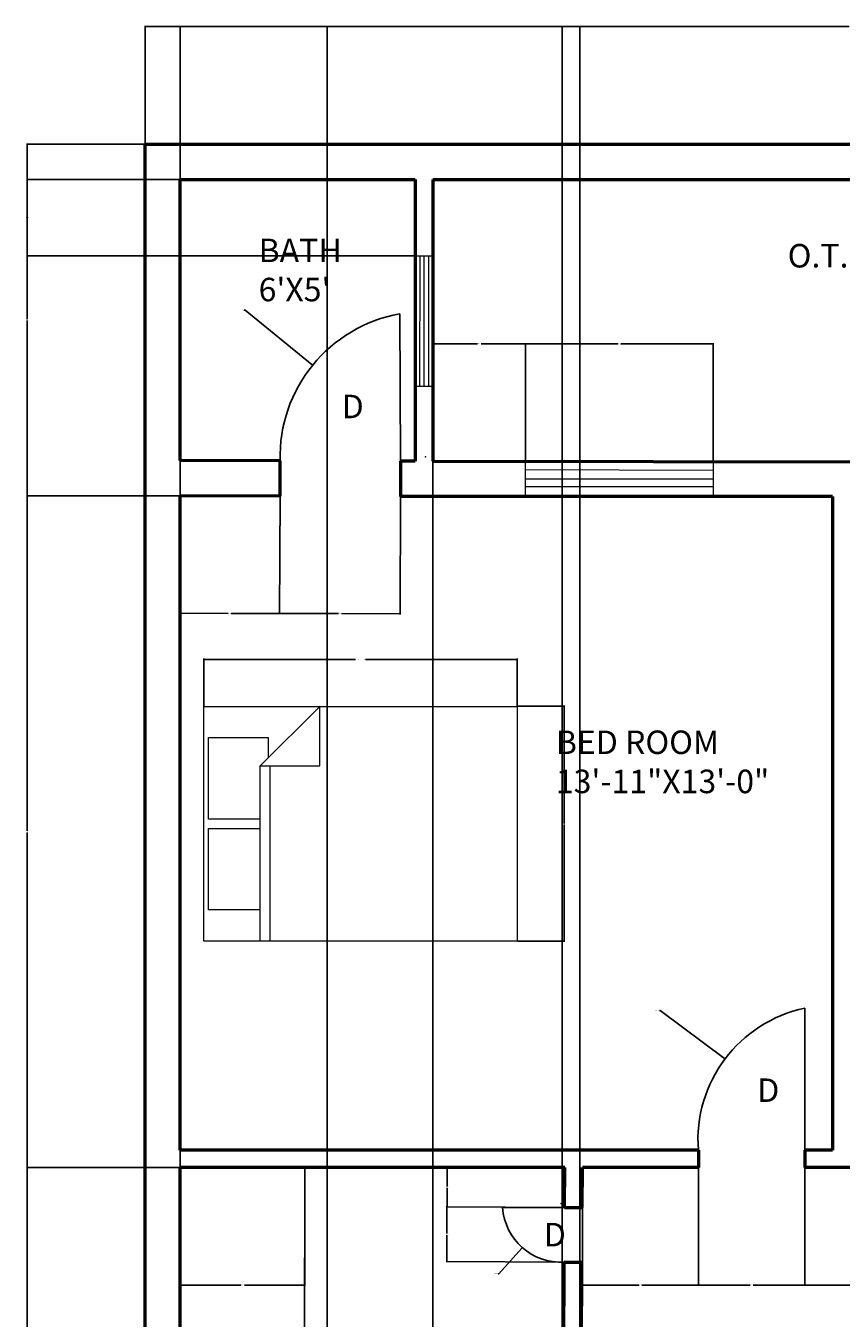
# Model space of a CAD drawing. Units: inches. Extents: x 2341 to 2761, y 2129 to 2789.
# Tile 3 of 4: x 2341 to 2549, y 2459 to 2789. Entities that reach past the tile are written whole.
import ezdxf

# ---------------------------------------------------------------- set-up
doc = ezdxf.new("R2010")
doc.units = ezdxf.units.IN
for name, color, linetype, lineweight in [('A-ANNO-DIMS', 2, 'Continuous', 18), ('A-ANNO-TEXT', 7, 'Continuous', 18), ('A-AREA-IDEN', 7, 'Continuous', 25), ('A-DOOR', 3, 'Continuous', 25), ('A-FLOR-FIXT', 9, 'Continuous', 25), ('A-FURN', 8, 'Continuous', 18), ('A-GLAZ', 4, 'Continuous', 18), ('A-WALL', 7, 'Continuous', 50)]:
    doc.layers.add(name, color=color, linetype=linetype, lineweight=lineweight)
doc.styles.get("Standard").update_dxf_attribs({"font": 'arial.ttf'})
doc.dimstyles.get("Standard").update_dxf_attribs({"dimtxt": 0.18, "dimasz": 0.18, "dimexe": 0.18, "dimexo": 0.0625, "dimgap": 0.09, "dimtad": 0, "dimtih": 1, "dimtoh": 1, "dimdec": 4, "dimzin": 0, "dimdsep": 46, "dimtxsty": 'Standard', "dimcen": 0.09, "dimadec": 0, "dimazin": 0, "dimtfac": 1, "dimtdec": 4, "dimtofl": 0, "dimtmove": 0, "dimatfit": 3, "dimfxl": 1, "dimtolj": 1, "dimtzin": 0, "dimarcsym": 0})

# ---------------------------------------------------------------- blocks, each defined once
blk = doc.blocks.new('Bed - Queen')
for p, q in [((0, -80.00003), (0, 0)), ((0, 0), (59.99999, 0)), ((59.99999, 0), (59.99999, -80.00003)), ((7.99999, -1.2), (28.79998, -1.2)), ((7.99999, -14.4), (7.99999, -1.2)), ((28.79998, -1.2), (28.79998, -14.4)), ((31.19999, -1.2), (51.99999, -1.2)), ((31.19999, -14.4), (31.19999, -1.2)), ((51.99999, -1.2), (51.99999, -16.4)), ((0, -14.4), (44.8, -14.4)), ((59.99999, -29.6), (44.8, -14.4)), ((44.8, -14.4), (44.8, -29.6)), ((51.99999, -16.4), (46.79936, -16.4)), ((44.8, -16.8), (0, -16.8)), ((44.8, -29.6), (59.99999, -29.6)), ((59.99999, -80.00003), (0, -80.00003))]:
    blk.add_line(p, q)
blk = doc.blocks.new('WIN-33IN-NARROW')
for p, q in [((0, 3.43), (33.34, 3.43)), ((0, 2.27), (33.34, 2.27)), ((0, 1.23), (33.34, 1.12))]:
    blk.add_line(p, q)
blk.add_lwpolyline([(0, 4.54), (33.34, 4.54), (33.34, 0), (0, 0)], close=True)
blk = doc.blocks.new('*D7')
at = {"layer": 'A-ANNO-DIMS', "color": 0, "lineweight": -2, "transparency": 16777216}
for p, q in [((2386.27, 2615.54), (2386.27, 2627.66)), ((2386.45, 2627.48), (2424.97, 2627.48)), ((2466.09, 2627.48), (2427.57, 2627.48)), ((2466.27, 2615.54), (2466.27, 2627.66))]:
    blk.add_line(p, q, dxfattribs=at)
at = {"layer": 'A-ANNO-DIMS', "color": 0, "transparency": 16777216}
for points in [[(2386.45, 2627.51), (2386.45, 2627.45), (2386.27, 2627.48)], [(2466.09, 2627.51), (2466.09, 2627.45), (2466.27, 2627.48)]]:
    blk.add_solid(points, dxfattribs=at)
at = {"layer": 'Defpoints', "color": 0, "transparency": 16777216}
for p in [(2386.27, 2627.48), (2386.27, 2615.48), (2466.27, 2615.48)]:
    blk.add_point(p, dxfattribs=at)
at = {"layer": 'A-ANNO-DIMS', "color": 0, "transparency": 16777216, "insert": (2426.27, 2627.48), "char_height": 0.18, "attachment_point": 5}
blk.add_mtext('\\A1;QUEEN BED 80 TYP.', dxfattribs=at)
blk = doc.blocks.new('*D8')
at = {"layer": 'A-ANNO-DIMS', "color": 0, "lineweight": -2, "transparency": 16777216}
for p, q in [((2466.33, 2615.48), (2478.45, 2615.48)), ((2478.27, 2615.3), (2478.27, 2585.66)), ((2478.27, 2555.66), (2478.27, 2585.3)), ((2466.33, 2555.48), (2478.45, 2555.48))]:
    blk.add_line(p, q, dxfattribs=at)
at = {"layer": 'A-ANNO-DIMS', "color": 0, "transparency": 16777216}
for points in [[(2478.24, 2615.3), (2478.3, 2615.3), (2478.27, 2615.48)], [(2478.24, 2555.66), (2478.3, 2555.66), (2478.27, 2555.48)]]:
    blk.add_solid(points, dxfattribs=at)
at = {"layer": 'Defpoints', "color": 0, "transparency": 16777216}
for p in [(2466.27, 2615.48), (2478.27, 2615.48), (2466.27, 2555.48)]:
    blk.add_point(p, dxfattribs=at)
at = {"layer": 'A-ANNO-DIMS', "color": 0, "transparency": 16777216, "insert": (2478.27, 2585.48), "char_height": 0.18, "attachment_point": 5}
blk.add_mtext('\\A1;60 TYP.', dxfattribs=at)
blk = doc.blocks.new('*D11')
at = {"layer": 'A-ANNO-DIMS', "color": 0, "lineweight": -2, "transparency": 16777216}
for p, q in [((2371.24, 2759.18), (2371.24, 2789.36)), ((2371.42, 2789.18), (2550.95, 2789.18)), ((2731.06, 2789.18), (2551.53, 2789.18)), ((2731.24, 2759.18), (2731.24, 2789.36))]:
    blk.add_line(p, q, dxfattribs=at)
at = {"layer": 'A-ANNO-DIMS', "color": 0, "transparency": 16777216}
for points in [[(2371.42, 2789.21), (2371.42, 2789.15), (2371.24, 2789.18)], [(2731.06, 2789.21), (2731.06, 2789.15), (2731.24, 2789.18)]]:
    blk.add_solid(points, dxfattribs=at)
at = {"layer": 'Defpoints', "color": 0, "transparency": 16777216}
for p in [(2731.24, 2789.18), (2371.24, 2759.12), (2731.24, 2759.12)]:
    blk.add_point(p, dxfattribs=at)
at = {"layer": 'A-ANNO-DIMS', "color": 0, "transparency": 16777216, "insert": (2551.24, 2789.18), "char_height": 0.18, "attachment_point": 5}
blk.add_mtext('\\A1;360', dxfattribs=at)
blk = doc.blocks.new('*D14')
at = {"layer": 'A-ANNO-DIMS', "color": 0, "lineweight": -2, "transparency": 16777216}
for p, q in [((2380.18, 2497.6), (2341.01, 2497.6)), ((2341.19, 2497.42), (2341.19, 2419.77)), ((2341.19, 2341.76), (2341.19, 2419.4)), ((2380.18, 2341.58), (2341.01, 2341.58))]:
    blk.add_line(p, q, dxfattribs=at)
at = {"layer": 'A-ANNO-DIMS', "color": 0, "transparency": 16777216}
for points in [[(2341.16, 2497.42), (2341.22, 2497.42), (2341.19, 2497.6)], [(2341.16, 2341.76), (2341.22, 2341.76), (2341.19, 2341.58)]]:
    blk.add_solid(points, dxfattribs=at)
at = {"layer": 'Defpoints', "color": 0, "transparency": 16777216}
for p in [(2341.19, 2497.6), (2380.24, 2497.6), (2380.24, 2341.58)]:
    blk.add_point(p, dxfattribs=at)
at = {"layer": 'A-ANNO-DIMS', "color": 0, "transparency": 16777216, "insert": (2341.19, 2419.59), "char_height": 0.18, "attachment_point": 5}
blk.add_mtext('\\A1;156.02', dxfattribs=at)
blk = doc.blocks.new('*D15')
at = {"layer": 'A-ANNO-DIMS', "color": 0, "lineweight": -2, "transparency": 16777216}
for p, q in [((2380.18, 2669.3), (2341.01, 2669.3)), ((2341.19, 2669.12), (2341.19, 2583.63)), ((2341.19, 2497.78), (2341.19, 2583.27)), ((2380.18, 2497.6), (2341.01, 2497.6))]:
    blk.add_line(p, q, dxfattribs=at)
at = {"layer": 'A-ANNO-DIMS', "color": 0, "transparency": 16777216}
for points in [[(2341.16, 2669.12), (2341.22, 2669.12), (2341.19, 2669.3)], [(2341.16, 2497.78), (2341.22, 2497.78), (2341.19, 2497.6)]]:
    blk.add_solid(points, dxfattribs=at)
at = {"layer": 'Defpoints', "color": 0, "transparency": 16777216}
for p in [(2341.19, 2669.3), (2380.24, 2669.3), (2380.24, 2497.6)]:
    blk.add_point(p, dxfattribs=at)
at = {"layer": 'A-ANNO-DIMS', "color": 0, "transparency": 16777216, "insert": (2341.19, 2583.45), "char_height": 0.18, "attachment_point": 5}
blk.add_mtext('\\A1;171.7', dxfattribs=at)
blk = doc.blocks.new('*D16')
at = {"layer": 'A-ANNO-DIMS', "color": 0, "lineweight": -2, "transparency": 16777216}
for p, q in [((2371.18, 2759.12), (2341.01, 2759.12)), ((2341.19, 2758.94), (2341.19, 2714.39)), ((2341.19, 2669.48), (2341.19, 2714.03)), ((2380.18, 2669.3), (2341.01, 2669.3))]:
    blk.add_line(p, q, dxfattribs=at)
at = {"layer": 'A-ANNO-DIMS', "color": 0, "transparency": 16777216}
for points in [[(2341.16, 2758.94), (2341.22, 2758.94), (2341.19, 2759.12)], [(2341.16, 2669.48), (2341.22, 2669.48), (2341.19, 2669.3)]]:
    blk.add_solid(points, dxfattribs=at)
at = {"layer": 'Defpoints', "color": 0, "transparency": 16777216}
for p in [(2341.19, 2759.12), (2371.24, 2759.12), (2380.24, 2669.3)]:
    blk.add_point(p, dxfattribs=at)
at = {"layer": 'A-ANNO-DIMS', "color": 0, "transparency": 16777216, "insert": (2341.19, 2714.21), "char_height": 0.18, "attachment_point": 5}
blk.add_mtext('\\A1;89.82', dxfattribs=at)
blk = doc.blocks.new('*D17')
at = {"layer": 'A-ANNO-DIMS', "color": 0, "lineweight": -2, "transparency": 16777216}
for p, q in [((2444.74, 2750.05), (2444.74, 2128.92)), ((2658.39, 2749.97), (2658.39, 2128.92)), ((2444.92, 2129.1), (2551.1, 2129.1)), ((2658.21, 2129.1), (2552.03, 2129.1))]:
    blk.add_line(p, q, dxfattribs=at)
at = {"layer": 'A-ANNO-DIMS', "color": 0, "transparency": 16777216}
for points in [[(2444.92, 2129.13), (2444.92, 2129.07), (2444.74, 2129.1)], [(2658.21, 2129.13), (2658.21, 2129.07), (2658.39, 2129.1)]]:
    blk.add_solid(points, dxfattribs=at)
at = {"layer": 'Defpoints', "color": 0, "transparency": 16777216}
for p in [(2444.74, 2750.12), (2658.39, 2750.04), (2658.39, 2129.1)]:
    blk.add_point(p, dxfattribs=at)
at = {"layer": 'A-ANNO-DIMS', "color": 0, "transparency": 16777216, "insert": (2551.56, 2129.1), "char_height": 0.18, "attachment_point": 5}
blk.add_mtext('\\A1;213.65', dxfattribs=at)
blk = doc.blocks.new('*D28')
at = {"layer": 'A-ANNO-DIMS', "color": 0, "lineweight": -2, "transparency": 16777216}
for p, q in [((2477.74, 2346.18), (2477.74, 2789.36)), ((2477.92, 2789.18), (2479.73, 2789.18)), ((2482.06, 2789.18), (2480.25, 2789.18)), ((2482.24, 2346.16), (2482.24, 2789.36))]:
    blk.add_line(p, q, dxfattribs=at)
at = {"layer": 'A-ANNO-DIMS', "color": 0, "transparency": 16777216}
for points in [[(2477.92, 2789.21), (2477.92, 2789.15), (2477.74, 2789.18)], [(2482.06, 2789.21), (2482.06, 2789.15), (2482.24, 2789.18)]]:
    blk.add_solid(points, dxfattribs=at)
at = {"layer": 'Defpoints', "color": 0, "transparency": 16777216}
for p in [(2482.24, 2789.18), (2477.74, 2346.12), (2482.24, 2346.1)]:
    blk.add_point(p, dxfattribs=at)
at = {"layer": 'A-ANNO-DIMS', "color": 0, "transparency": 16777216, "insert": (2479.99, 2789.18), "char_height": 0.18, "attachment_point": 5}
blk.add_mtext('\\A1;4.5', dxfattribs=at)
blk = doc.blocks.new('*D29')
at = {"layer": 'A-ANNO-DIMS', "color": 0, "lineweight": -2, "transparency": 16777216}
for p, q in [((2371.24, 2759.06), (2371.24, 2128.92)), ((2380.24, 2750.06), (2380.24, 2128.92)), ((2371.42, 2129.1), (2375.59, 2129.1)), ((2380.06, 2129.1), (2375.89, 2129.1))]:
    blk.add_line(p, q, dxfattribs=at)
at = {"layer": 'A-ANNO-DIMS', "color": 0, "transparency": 16777216}
for points in [[(2371.42, 2129.13), (2371.42, 2129.07), (2371.24, 2129.1)], [(2380.06, 2129.13), (2380.06, 2129.07), (2380.24, 2129.1)]]:
    blk.add_solid(points, dxfattribs=at)
at = {"layer": 'Defpoints', "color": 0, "transparency": 16777216}
for p in [(2371.24, 2759.12), (2380.24, 2750.12), (2380.24, 2129.1)]:
    blk.add_point(p, dxfattribs=at)
at = {"layer": 'A-ANNO-DIMS', "color": 0, "transparency": 16777216, "insert": (2375.74, 2129.1), "char_height": 0.18, "attachment_point": 5}
blk.add_mtext('\\A1;9', dxfattribs=at)
blk = doc.blocks.new('*D31')
at = {"layer": 'A-ANNO-DIMS', "color": 0, "lineweight": -2, "transparency": 16777216}
for p, q in [((2444.74, 2678.18), (2444.78, 2708.32)), ((2444.96, 2708.14), (2456.13, 2708.12)), ((2468.24, 2708.11), (2457.06, 2708.12)), ((2468.39, 2678.15), (2468.42, 2708.29))]:
    blk.add_line(p, q, dxfattribs=at)
at = {"layer": 'A-ANNO-DIMS', "color": 0, "transparency": 16777216}
for points in [[(2444.96, 2708.17), (2444.96, 2708.11), (2444.78, 2708.14)], [(2468.24, 2708.14), (2468.24, 2708.08), (2468.42, 2708.11)]]:
    blk.add_solid(points, dxfattribs=at)
at = {"layer": 'Defpoints', "color": 0, "transparency": 16777216}
for p in [(2468.42, 2708.11), (2444.74, 2678.12), (2468.39, 2678.09)]:
    blk.add_point(p, dxfattribs=at)
at = {"layer": 'A-ANNO-DIMS', "color": 0, "transparency": 16777216, "insert": (2456.6, 2708.12), "char_height": 0.18, "attachment_point": 5}
blk.add_mtext('\\A1;23.643', dxfattribs=at)
blk = doc.blocks.new('*D32')
at = {"layer": 'A-ANNO-DIMS', "color": 0, "lineweight": -2, "transparency": 16777216}
for p, q in [((2468.39, 2678.15), (2468.39, 2708.29)), ((2468.57, 2708.11), (2491.95, 2708.11)), ((2516.12, 2708.11), (2492.74, 2708.11)), ((2516.3, 2678.15), (2516.3, 2708.29))]:
    blk.add_line(p, q, dxfattribs=at)
at = {"layer": 'A-ANNO-DIMS', "color": 0, "transparency": 16777216}
for points in [[(2468.57, 2708.14), (2468.57, 2708.08), (2468.39, 2708.11)], [(2516.12, 2708.14), (2516.12, 2708.08), (2516.3, 2708.11)]]:
    blk.add_solid(points, dxfattribs=at)
at = {"layer": 'Defpoints', "color": 0, "transparency": 16777216}
for p in [(2516.3, 2708.11), (2468.39, 2678.09), (2516.3, 2678.09)]:
    blk.add_point(p, dxfattribs=at)
at = {"layer": 'A-ANNO-DIMS', "color": 0, "transparency": 16777216, "insert": (2492.34, 2708.11), "char_height": 0.18, "attachment_point": 5}
blk.add_mtext('\\A1;47.92', dxfattribs=at)
blk = doc.blocks.new('*D33')
at = {"layer": 'A-ANNO-DIMS', "color": 0, "lineweight": -2, "transparency": 16777216}
for p, q in [((2380.24, 2346.14), (2380.24, 2789.36)), ((2380.42, 2789.18), (2398.59, 2789.18)), ((2417.55, 2789.18), (2399.38, 2789.18)), ((2417.73, 2346.19), (2417.73, 2789.36))]:
    blk.add_line(p, q, dxfattribs=at)
at = {"layer": 'A-ANNO-DIMS', "color": 0, "transparency": 16777216}
for points in [[(2380.42, 2789.21), (2380.42, 2789.15), (2380.24, 2789.18)], [(2417.55, 2789.21), (2417.55, 2789.15), (2417.73, 2789.18)]]:
    blk.add_solid(points, dxfattribs=at)
at = {"layer": 'Defpoints', "color": 0, "transparency": 16777216}
for p in [(2417.73, 2789.18), (2380.24, 2346.08), (2417.73, 2346.13)]:
    blk.add_point(p, dxfattribs=at)
at = {"layer": 'A-ANNO-DIMS', "color": 0, "transparency": 16777216, "insert": (2398.99, 2789.18), "char_height": 0.18, "attachment_point": 5}
blk.add_mtext('\\A1;37.49', dxfattribs=at)
blk = doc.blocks.new('*D36')
at = {"layer": 'A-ANNO-DIMS', "color": 0, "lineweight": -2, "transparency": 16777216}
for p, q in [((2440.18, 2750.12), (2341.01, 2750.12)), ((2341.19, 2749.94), (2341.19, 2740.52)), ((2341.19, 2730.74), (2341.19, 2740.16)), ((2440.14, 2730.56), (2341.01, 2730.56))]:
    blk.add_line(p, q, dxfattribs=at)
at = {"layer": 'A-ANNO-DIMS', "color": 0, "transparency": 16777216}
for points in [[(2341.16, 2749.94), (2341.22, 2749.94), (2341.19, 2750.12)], [(2341.16, 2730.74), (2341.22, 2730.74), (2341.19, 2730.56)]]:
    blk.add_solid(points, dxfattribs=at)
at = {"layer": 'Defpoints', "color": 0, "transparency": 16777216}
for p in [(2341.19, 2750.12), (2440.24, 2750.12), (2440.2, 2730.56)]:
    blk.add_point(p, dxfattribs=at)
at = {"layer": 'A-ANNO-DIMS', "color": 0, "transparency": 16777216, "insert": (2341.19, 2740.34), "char_height": 0.18, "attachment_point": 5}
blk.add_mtext('\\A1;19.554', dxfattribs=at)
blk = doc.blocks.new('*D37')
at = {"layer": 'A-ANNO-DIMS', "color": 0, "lineweight": -2, "transparency": 16777216}
for p, q in [((2380.24, 2669.24), (2380.15, 2639.1)), ((2405.71, 2669.16), (2405.62, 2639.02)), ((2380.33, 2639.28), (2392.49, 2639.24)), ((2405.44, 2639.2), (2393.28, 2639.24))]:
    blk.add_line(p, q, dxfattribs=at)
at = {"layer": 'A-ANNO-DIMS', "color": 0, "transparency": 16777216}
for points in [[(2380.33, 2639.31), (2380.33, 2639.25), (2380.15, 2639.28)], [(2405.44, 2639.23), (2405.44, 2639.17), (2405.62, 2639.2)]]:
    blk.add_solid(points, dxfattribs=at)
at = {"layer": 'Defpoints', "color": 0, "transparency": 16777216}
for p in [(2380.24, 2669.3), (2405.71, 2669.22), (2380.15, 2639.28)]:
    blk.add_point(p, dxfattribs=at)
at = {"layer": 'A-ANNO-DIMS', "color": 0, "transparency": 16777216, "insert": (2392.89, 2639.24), "char_height": 0.18, "attachment_point": 5}
blk.add_mtext('\\A1;25.47', dxfattribs=at)
blk = doc.blocks.new('*D38')
at = {"layer": 'A-ANNO-DIMS', "color": 0, "lineweight": -2, "transparency": 16777216}
for p, q in [((2405.71, 2669.16), (2405.62, 2639.02)), ((2436.5, 2669.07), (2436.41, 2638.93)), ((2405.8, 2639.2), (2420.62, 2639.16)), ((2436.23, 2639.11), (2421.41, 2639.16))]:
    blk.add_line(p, q, dxfattribs=at)
at = {"layer": 'A-ANNO-DIMS', "color": 0, "transparency": 16777216}
for points in [[(2405.8, 2639.23), (2405.8, 2639.17), (2405.62, 2639.2)], [(2436.23, 2639.14), (2436.23, 2639.08), (2436.41, 2639.11)]]:
    blk.add_solid(points, dxfattribs=at)
at = {"layer": 'Defpoints', "color": 0, "transparency": 16777216}
for p in [(2405.71, 2669.22), (2436.5, 2669.13), (2405.62, 2639.2)]:
    blk.add_point(p, dxfattribs=at)
at = {"layer": 'A-ANNO-DIMS', "color": 0, "transparency": 16777216, "insert": (2421.02, 2639.16), "char_height": 0.18, "attachment_point": 5}
blk.add_mtext('\\A1;30.79', dxfattribs=at)
blk = doc.blocks.new('*D43')
at = {"layer": 'A-ANNO-DIMS', "color": 0, "lineweight": -2, "transparency": 16777216}
for p, q in [((2482.91, 2497.53), (2482.91, 2467.4)), ((2512.53, 2497.53), (2512.53, 2467.4)), ((2483.09, 2467.58), (2497.33, 2467.58)), ((2512.35, 2467.58), (2498.11, 2467.58))]:
    blk.add_line(p, q, dxfattribs=at)
at = {"layer": 'A-ANNO-DIMS', "color": 0, "transparency": 16777216}
for points in [[(2483.09, 2467.61), (2483.09, 2467.55), (2482.91, 2467.58)], [(2512.35, 2467.61), (2512.35, 2467.55), (2512.53, 2467.58)]]:
    blk.add_solid(points, dxfattribs=at)
at = {"layer": 'Defpoints', "color": 0, "transparency": 16777216}
for p in [(2482.91, 2497.6), (2512.53, 2497.6), (2482.91, 2467.58)]:
    blk.add_point(p, dxfattribs=at)
at = {"layer": 'A-ANNO-DIMS', "color": 0, "transparency": 16777216, "insert": (2497.72, 2467.58), "char_height": 0.18, "attachment_point": 5}
blk.add_mtext('\\A1;29.62', dxfattribs=at)
blk = doc.blocks.new('*D44')
at = {"layer": 'A-ANNO-DIMS', "color": 0, "lineweight": -2, "transparency": 16777216}
for p, q in [((2512.53, 2497.53), (2512.53, 2467.4)), ((2539.74, 2497.53), (2539.74, 2467.4)), ((2512.71, 2467.58), (2525.76, 2467.58)), ((2539.56, 2467.58), (2526.51, 2467.58))]:
    blk.add_line(p, q, dxfattribs=at)
at = {"layer": 'A-ANNO-DIMS', "color": 0, "transparency": 16777216}
for points in [[(2512.71, 2467.61), (2512.71, 2467.55), (2512.53, 2467.58)], [(2539.56, 2467.61), (2539.56, 2467.55), (2539.74, 2467.58)]]:
    blk.add_solid(points, dxfattribs=at)
at = {"layer": 'Defpoints', "color": 0, "transparency": 16777216}
for p in [(2512.53, 2497.6), (2539.74, 2497.6), (2512.53, 2467.58)]:
    blk.add_point(p, dxfattribs=at)
at = {"layer": 'A-ANNO-DIMS', "color": 0, "transparency": 16777216, "insert": (2526.13, 2467.58), "char_height": 0.18, "attachment_point": 5}
blk.add_mtext('\\A1;27.21', dxfattribs=at)
blk = doc.blocks.new('*D45')
at = {"layer": 'A-ANNO-DIMS', "color": 0, "lineweight": -2, "transparency": 16777216}
for p, q in [((2539.74, 2497.53), (2539.74, 2467.4)), ((2567.7, 2497.53), (2567.7, 2467.4)), ((2539.92, 2467.58), (2553.25, 2467.58)), ((2567.52, 2467.58), (2554.19, 2467.58))]:
    blk.add_line(p, q, dxfattribs=at)
at = {"layer": 'A-ANNO-DIMS', "color": 0, "transparency": 16777216}
for points in [[(2539.92, 2467.61), (2539.92, 2467.55), (2539.74, 2467.58)], [(2567.52, 2467.61), (2567.52, 2467.55), (2567.7, 2467.58)]]:
    blk.add_solid(points, dxfattribs=at)
at = {"layer": 'Defpoints', "color": 0, "transparency": 16777216}
for p in [(2539.74, 2497.6), (2567.7, 2497.6), (2539.74, 2467.58)]:
    blk.add_point(p, dxfattribs=at)
at = {"layer": 'A-ANNO-DIMS', "color": 0, "transparency": 16777216, "insert": (2553.72, 2467.58), "char_height": 0.18, "attachment_point": 5}
blk.add_mtext('\\A1;27.967', dxfattribs=at)
blk = doc.blocks.new('*D47')
at = {"layer": 'A-ANNO-DIMS', "color": 0, "lineweight": -2, "transparency": 16777216}
for p, q in [((2478.3, 2487.42), (2448.17, 2487.56)), ((2448.34, 2487.37), (2448.32, 2480.75)), ((2448.28, 2473.77), (2448.31, 2480.39)), ((2478.24, 2473.45), (2448.1, 2473.59))]:
    blk.add_line(p, q, dxfattribs=at)
at = {"layer": 'A-ANNO-DIMS', "color": 0, "transparency": 16777216}
for points in [[(2448.31, 2487.37), (2448.37, 2487.37), (2448.35, 2487.55)], [(2448.25, 2473.77), (2448.31, 2473.77), (2448.28, 2473.59)]]:
    blk.add_solid(points, dxfattribs=at)
at = {"layer": 'Defpoints', "color": 0, "transparency": 16777216}
for p in [(2448.35, 2487.55), (2478.37, 2487.42), (2478.3, 2473.45)]:
    blk.add_point(p, dxfattribs=at)
at = {"layer": 'A-ANNO-DIMS', "color": 0, "transparency": 16777216, "insert": (2448.31, 2480.57), "char_height": 0.18, "attachment_point": 5}
blk.add_mtext('\\A1;13.968', dxfattribs=at)
blk = doc.blocks.new('*D48')
at = {"layer": 'A-ANNO-DIMS', "color": 0, "lineweight": -2, "transparency": 16777216}
for p, q in [((2478.35, 2497.6), (2448.21, 2497.73)), ((2448.39, 2497.55), (2448.37, 2492.82)), ((2448.35, 2487.73), (2448.37, 2492.46)), ((2478.3, 2487.42), (2448.17, 2487.56))]:
    blk.add_line(p, q, dxfattribs=at)
at = {"layer": 'A-ANNO-DIMS', "color": 0, "transparency": 16777216}
for points in [[(2448.36, 2497.55), (2448.42, 2497.55), (2448.39, 2497.73)], [(2448.32, 2487.73), (2448.38, 2487.73), (2448.35, 2487.55)]]:
    blk.add_solid(points, dxfattribs=at)
at = {"layer": 'Defpoints', "color": 0, "transparency": 16777216}
for p in [(2448.39, 2497.73), (2478.41, 2497.6), (2478.37, 2487.42)]:
    blk.add_point(p, dxfattribs=at)
at = {"layer": 'A-ANNO-DIMS', "color": 0, "transparency": 16777216, "insert": (2448.37, 2492.64), "char_height": 0.18, "attachment_point": 5}
blk.add_mtext('\\A1;10.175', dxfattribs=at)
blk = doc.blocks.new('*D58')
at = {"layer": 'A-ANNO-DIMS', "color": 0, "lineweight": -2, "transparency": 16777216}
for p, q in [((2380.24, 2497.53), (2380.24, 2467.4)), ((2412.09, 2497.53), (2412.09, 2467.4)), ((2380.42, 2467.58), (2395.7, 2467.58)), ((2411.91, 2467.58), (2396.63, 2467.58))]:
    blk.add_line(p, q, dxfattribs=at)
at = {"layer": 'A-ANNO-DIMS', "color": 0, "transparency": 16777216}
for points in [[(2380.42, 2467.61), (2380.42, 2467.55), (2380.24, 2467.58)], [(2411.91, 2467.61), (2411.91, 2467.55), (2412.09, 2467.58)]]:
    blk.add_solid(points, dxfattribs=at)
at = {"layer": 'Defpoints', "color": 0, "transparency": 16777216}
for p in [(2380.24, 2497.6), (2412.09, 2497.6), (2380.24, 2467.58)]:
    blk.add_point(p, dxfattribs=at)
at = {"layer": 'A-ANNO-DIMS', "color": 0, "transparency": 16777216, "insert": (2396.16, 2467.58), "char_height": 0.18, "attachment_point": 5}
blk.add_mtext('\\A1;31.845', dxfattribs=at)
blk = doc.blocks.new('*D67')
at = {"layer": 'A-ANNO-DIMS', "color": 0, "lineweight": -2, "transparency": 16777216}
for p, q in [((2396.6, 2716.74), (2396.78, 2716.74)), ((2396.78, 2716.74), (2413.93, 2702.78)), ((2442.8, 2679.21), (2442.98, 2679.21)), ((2442.89, 2679.12), (2442.89, 2679.3))]:
    blk.add_line(p, q, dxfattribs=at)
at = {"layer": 'A-ANNO-DIMS', "color": 0, "transparency": 16777216}
blk.add_solid([(2413.95, 2702.81), (2413.91, 2702.76), (2414.07, 2702.67)], dxfattribs=at)
at = {"layer": 'Defpoints', "color": 0, "transparency": 16777216}
for p in [(2414.07, 2702.67), (2442.89, 2679.21)]:
    blk.add_point(p, dxfattribs=at)
at = {"layer": 'A-ANNO-DIMS', "color": 0, "transparency": 16777216, "insert": (2396.12, 2716.74), "char_height": 0.18, "attachment_point": 5}
blk.add_mtext('\\A1;R37.16', dxfattribs=at)
blk = doc.blocks.new('*D69')
at = {"layer": 'A-ANNO-DIMS', "color": 0, "lineweight": -2, "transparency": 16777216}
for p, q in [((2502.64, 2537.72), (2502.82, 2537.72)), ((2502.82, 2537.72), (2519.17, 2525.45)), ((2546.71, 2504.71), (2546.89, 2504.71)), ((2546.8, 2504.62), (2546.8, 2504.8))]:
    blk.add_line(p, q, dxfattribs=at)
at = {"layer": 'A-ANNO-DIMS', "color": 0, "transparency": 16777216}
blk.add_solid([(2519.19, 2525.47), (2519.15, 2525.42), (2519.31, 2525.34)], dxfattribs=at)
at = {"layer": 'Defpoints', "color": 0, "transparency": 16777216}
for p in [(2519.31, 2525.34), (2546.8, 2504.71)]:
    blk.add_point(p, dxfattribs=at)
at = {"layer": 'A-ANNO-DIMS', "color": 0, "transparency": 16777216, "insert": (2502.09, 2537.72), "char_height": 0.18, "attachment_point": 5}
blk.add_mtext('\\A1;R34.375', dxfattribs=at)
blk = doc.blocks.new('*D74')
at = {"layer": 'A-ANNO-DIMS', "color": 0, "lineweight": -2, "transparency": 16777216}
for p, q in [((2477.4, 2488.4), (2477.58, 2488.4)), ((2477.49, 2488.31), (2477.49, 2488.49)), ((2461.6, 2470.48), (2467.44, 2477.06)), ((2461.42, 2470.48), (2461.6, 2470.48))]:
    blk.add_line(p, q, dxfattribs=at)
at = {"layer": 'A-ANNO-DIMS', "color": 0, "transparency": 16777216}
blk.add_solid([(2467.41, 2477.08), (2467.46, 2477.04), (2467.56, 2477.2)], dxfattribs=at)
at = {"layer": 'Defpoints', "color": 0, "transparency": 16777216}
for p in [(2477.49, 2488.4), (2467.56, 2477.2)]:
    blk.add_point(p, dxfattribs=at)
at = {"layer": 'A-ANNO-DIMS', "color": 0, "transparency": 16777216, "insert": (2460.87, 2470.48), "char_height": 0.18, "attachment_point": 5}
blk.add_mtext('\\A1;R14.968', dxfattribs=at)

msp = doc.modelspace()

# ---------------------------------------------------------------- linework, layer by layer
at = {"layer": 'A-DOOR'}
for p, q in [((2436.4665, 2678.1289), (2436.312, 2715.7849)), ((2539.7368, 2502.0958), (2539.7368, 2538.3463)), ((2478.3651, 2487.4212), (2462.5493, 2487.4212))]:
    msp.add_line(p, q, dxfattribs=at)
for centre, radius, start, end in [((2442.8885, 2679.2119), 37.1596, 100.193859, 181.524002), ((2546.8043, 2504.7061), 34.3746, 101.864921, 184.355124), ((2477.4854, 2488.3993), 14.9682, 183.74658, 273.131619)]:
    msp.add_arc(centre, radius, start, end, dxfattribs=at)
at = {"layer": 'A-FLOR-FIXT'}
msp.add_line((2411.7316, 2378.3809), (2412.0874, 2497.5958), dxfattribs=at)
at = {"layer": 'A-GLAZ'}
for p, q in [((2468.3855, 2676.0036), (2516.3027, 2675.8169)), ((2468.3855, 2673.5973), (2516.3027, 2673.5973)), ((2468.3855, 2671.617), (2516.3027, 2671.617))]:
    msp.add_line(p, q, dxfattribs=at)
msp.add_lwpolyline([(2468.3855, 2678.0911), (2516.3027, 2678.0911), (2516.3027, 2669.1034), (2468.3855, 2669.1034)], close=True, dxfattribs=at)
at = {"layer": 'A-WALL'}
for p, q in [((2371.242, 2759.1219), (2731.242, 2759.1219)), ((2371.242, 2159.1219), (2371.242, 2759.1219)), ((2380.242, 2750.1219), (2440.242, 2750.1173)), ((2380.242, 2678.3021), (2380.242, 2750.1219)), ((2440.242, 2750.1173), (2440.242, 2678.1173)), ((2444.742, 2750.1173), (2444.742, 2678.1173)), ((2444.742, 2750.1173), (2658.3873, 2750.0366)), ((2405.742, 2678.2236), (2380.242, 2678.3021)), ((2405.7143, 2669.2236), (2405.742, 2678.2236)), ((2440.242, 2678.1173), (2436.4665, 2678.1289)), ((2436.4665, 2678.1289), (2436.5035, 2669.1288)), ((2444.742, 2678.1173), (2563.3637, 2677.9857)), ((2371.242, 2669.3298), (2371.2143, 2669.3299)), ((2405.7143, 2669.2236), (2380.242, 2669.3021)), ((2380.242, 2502.0958), (2380.242, 2669.3021)), ((2440.2143, 2669.1173), (2436.5035, 2669.1288)), ((2546.742, 2669.0958), (2438.3589, 2669.1231)), ((2546.742, 2669.0958), (2546.742, 2502.0958)), ((2512.529, 2502.0958), (2380.242, 2502.0958)), ((2478.4303, 2502.0958), (2478.4304, 2502.1158)), ((2512.529, 2502.0958), (2512.529, 2497.5958)), ((2546.742, 2502.0958), (2539.7368, 2502.0958)), ((2539.7368, 2502.0958), (2539.7368, 2497.5958)), ((2478.4103, 2497.5958), (2380.242, 2497.5958)), ((2380.242, 2346.0773), (2380.242, 2497.5958)), ((2478.3651, 2487.4212), (2478.4103, 2497.5958)), ((2482.8652, 2487.4212), (2482.9104, 2497.5958)), ((2512.529, 2497.5958), (2482.9104, 2497.5958)), ((2551.242, 2497.5958), (2539.7368, 2497.5958)), ((2478.3651, 2487.4212), (2482.8652, 2487.4212)), ((2477.7379, 2346.1158), (2478.3031, 2473.4534)), ((2478.3031, 2473.4534), (2482.8032, 2473.4534)), ((2482.2379, 2346.0958), (2482.8032, 2473.4534))]:
    msp.add_line(p, q, dxfattribs=at)

# ---------------------------------------------------------------- block references
at = {"layer": 'A-FURN', "rotation": 90}
msp.add_blockref('Bed - Queen', (2386.271, 2555.4785), dxfattribs=at)
at = {"layer": 'A-GLAZ', "rotation": 270.0000000000046}
msp.add_blockref('WIN-33IN-NARROW', (2440.201, 2730.5633), dxfattribs=at)

# ---------------------------------------------------------------- texts
at = {"layer": 'A-ANNO-TEXT', "char_height": 6, "attachment_point": 1}
for insert in [(2421.4602, 2695.1014), (2527.5665, 2520.3944), (2473.0711, 2483.4817)]:
    msp.add_mtext_dynamic_manual_height_columns('D', width=9.002909, gutter_width=12.5, heights=[0], dxfattribs=dict(at, insert=insert))
at = {"layer": 'A-AREA-IDEN', "char_height": 6, "attachment_point": 1}
for s, width, insert in [("BATH \\P6'X5'", 22.746428, (2400.2491, 2734.9797)), ('O.T.S 5\'-5" WIDE ', 77.771128, (2535.3365, 2733.6222)), ('BED ROOM \\P13\'-11"X13\'-0"', 65.352086, (2476.1468, 2609.2925))]:
    msp.add_mtext_dynamic_manual_height_columns(s, width=width, gutter_width=12.5, heights=[0], dxfattribs=dict(at, insert=insert))

# ---------------------------------------------------------------- dimensions: what is measured, and where the dimension line sits
at = {"layer": 'A-ANNO-DIMS'}
for base, p1, p2, override, picture, middle in [((2731.242, 2789.1821), (2371.242, 2759.1219), (2731.242, 2759.1219), {"dimdec": 0, "dimlfac": 1, "dimrnd": 0, "dimzin": 0, "dimdsep": 46, "dimlunit": 2}, '*D11', (2551.242, 2789.1821)), ((2417.7307, 2789.1821), (2380.242, 2346.0773), (2417.7307, 2346.1252), {"dimdec": 2, "dimlfac": 1, "dimrnd": 0, "dimzin": 0, "dimdsep": 46, "dimlunit": 2}, '*D33', (2398.9864, 2789.1821)), ((2482.2379, 2789.1821), (2477.7379, 2346.1158), (2482.2379, 2346.0958), {"dimdec": 1, "dimlfac": 1, "dimrnd": 0, "dimzin": 0, "dimdsep": 46, "dimlunit": 2}, '*D28', (2479.9879, 2789.1821)), ((2380.242, 2129.1019), (2371.242, 2759.1219), (2380.242, 2750.1219), {"dimdec": 0, "dimlfac": 1, "dimrnd": 0, "dimzin": 0, "dimdsep": 46, "dimlunit": 2}, '*D29', (2375.742, 2129.1019)), ((2658.3873, 2129.1019), (2444.742, 2750.1173), (2658.3873, 2750.0366), {"dimdec": 2, "dimlfac": 1, "dimrnd": 0, "dimzin": 0, "dimdsep": 46, "dimlunit": 2}, '*D17', (2551.5646, 2129.1019)), ((2516.3027, 2708.1111), (2468.3855, 2678.0911), (2516.3027, 2678.0911), {"dimdec": 2, "dimlfac": 1, "dimrnd": 0, "dimzin": 0, "dimdsep": 46, "dimlunit": 2}, '*D32', (2492.3441, 2708.1111))]:
    dim = msp.add_linear_dim(base=base, p1=p1, p2=p2, dimstyle='Standard', override=override, dxfattribs=at)
    dim.commit()
    dim.dimension.update_dxf_attribs({"geometry": picture, "text_midpoint": middle})
for base, p1, p2, angle, override, picture, middle in [((2341.1943, 2759.1219), (2380.242, 2669.3021), (2371.242, 2759.1219), 90, {"dimdec": 2, "dimlfac": 1, "dimrnd": 0, "dimzin": 0, "dimdsep": 46, "dimlunit": 2}, '*D16', (2341.1943, 2714.212)), ((2341.19432, 2750.1173), (2440.20091, 2730.56376), (2440.24204, 2750.1173), 90, {"dimdec": 3, "dimlfac": 1, "dimrnd": 0, "dimzin": 0, "dimdsep": 46, "dimlunit": 2}, '*D36', (2341.19432, 2740.34053)), ((2468.4188, 2708.11105), (2444.74204, 2678.1173), (2468.3855, 2678.09107), 359.936454, {"dimdec": 3, "dimlfac": 1, "dimrnd": 0, "dimzin": 0, "dimdsep": 46, "dimlunit": 2}, '*D31', (2456.59707, 2708.12417)), ((2341.1943, 2669.3021), (2380.242, 2497.5958), (2380.242, 2669.3021), 90, {"dimdec": 1, "dimlfac": 1, "dimrnd": 0, "dimzin": 0, "dimdsep": 46, "dimlunit": 2}, '*D15', (2341.1943, 2583.4489)), ((2380.1496, 2639.2822), (2405.7143, 2669.2236), (2380.242, 2669.3021), 179.823499, {"dimdec": 2, "dimlfac": 1, "dimrnd": 0, "dimzin": 0, "dimdsep": 46, "dimlunit": 2}, '*D37', (2392.8857, 2639.243)), ((2405.6218, 2639.2038), (2436.5035, 2669.1288), (2405.7143, 2669.2236), 179.823499, {"dimdec": 2, "dimlfac": 1, "dimrnd": 0, "dimzin": 0, "dimdsep": 46, "dimlunit": 2}, '*D38', (2421.0164, 2639.1563)), ((2341.1943, 2497.5958), (2380.242, 2341.5773), (2380.242, 2497.5958), 90, {"dimdec": 2, "dimlfac": 1, "dimrnd": 0, "dimzin": 0, "dimdsep": 46, "dimlunit": 2}, '*D14', (2341.1943, 2419.5865)), ((2380.242, 2467.5758), (2412.0874, 2497.5958), (2380.242, 2497.5958), 180, {"dimdec": 3, "dimlfac": 1, "dimrnd": 0, "dimzin": 0, "dimdsep": 46, "dimlunit": 2}, '*D58', (2396.1647, 2467.5758)), ((2448.3906, 2497.729), (2478.3651, 2487.4212), (2478.4103, 2497.5958), 89.745684, {"dimdec": 3, "dimlfac": 1, "dimrnd": 0, "dimzin": 0, "dimdsep": 46, "dimlunit": 2}, '*D48', (2448.368, 2492.6417)), ((2482.9104, 2467.5758), (2512.529, 2497.5958), (2482.9104, 2497.5958), 180, {"dimdec": 2, "dimlfac": 1, "dimrnd": 0, "dimzin": 0, "dimdsep": 46, "dimlunit": 2}, '*D43', (2497.7197, 2467.5758)), ((2512.529, 2467.5758), (2539.7368, 2497.5958), (2512.529, 2497.5958), 180, {"dimdec": 2, "dimlfac": 1, "dimrnd": 0, "dimzin": 0, "dimdsep": 46, "dimlunit": 2}, '*D44', (2526.1329, 2467.5758)), ((2539.73676, 2467.57579), (2567.70327, 2497.59579), (2539.73676, 2497.59579), 180, {"dimdec": 3, "dimlfac": 1, "dimrnd": 0, "dimzin": 0, "dimdsep": 46, "dimlunit": 2}, '*D45', (2553.72001, 2467.57579)), ((2448.3454, 2487.5544), (2478.3031, 2473.4534), (2478.3651, 2487.4212), 89.745684, {"dimdec": 3, "dimlfac": 1, "dimrnd": 0, "dimzin": 0, "dimdsep": 46, "dimlunit": 2}, '*D47', (2448.3144, 2480.5706))]:
    dim = msp.add_linear_dim(base=base, p1=p1, p2=p2, angle=angle, dimstyle='Standard', override=override, dxfattribs=at)
    dim.commit()
    dim.dimension.update_dxf_attribs({"geometry": picture, "text_midpoint": middle})
for center, mpoint, override, picture, middle in [((2442.8885, 2679.2119), (2414.0677, 2702.6682), {"dimdec": 2, "dimlfac": 1, "dimrnd": 0, "dimzin": 0, "dimdsep": 46, "dimlunit": 2}, '*D67', (2396.1155, 2716.742)), ((2546.8043, 2504.7061), (2519.3122, 2525.3409), {"dimdec": 3, "dimlfac": 1, "dimrnd": 0, "dimzin": 0, "dimdsep": 46, "dimlunit": 2}, '*D69', (2502.0864, 2537.7217)), ((2477.4854, 2488.3993), (2467.5553, 2477.1993), {"dimdec": 3, "dimlfac": 1, "dimrnd": 0, "dimzin": 0, "dimdsep": 46, "dimlunit": 2}, '*D74', (2460.8673, 2470.4794))]:
    dim = msp.add_radius_dim(center=center, mpoint=mpoint, dimstyle='Standard', override=override, dxfattribs=at)
    dim.commit()
    dim.dimension.update_dxf_attribs({"geometry": picture, "text_midpoint": middle, "dimtype": 164})
for base, p1, p2, angle, text, picture, middle in [((2386.271, 2627.4785), (2466.271, 2615.4784), (2386.271, 2615.4784), 180, 'QUEEN BED <> TYP.', '*D7', (2426.271, 2627.4785)), ((2478.271, 2615.4784), (2466.271, 2555.4785), (2466.271, 2615.4784), 90, '<> TYP.', '*D8', (2478.271, 2585.4785))]:
    dim = msp.add_linear_dim(base=base, p1=p1, p2=p2, angle=angle, text=text, dimstyle='Standard', override={"dimdec": 0, "dimlfac": 1, "dimrnd": 0, "dimzin": 0, "dimdsep": 46, "dimlunit": 2}, dxfattribs=at)
    dim.commit()
    dim.dimension.update_dxf_attribs({"geometry": picture, "text_midpoint": middle})

doc.saveas('drawing.dxf')
